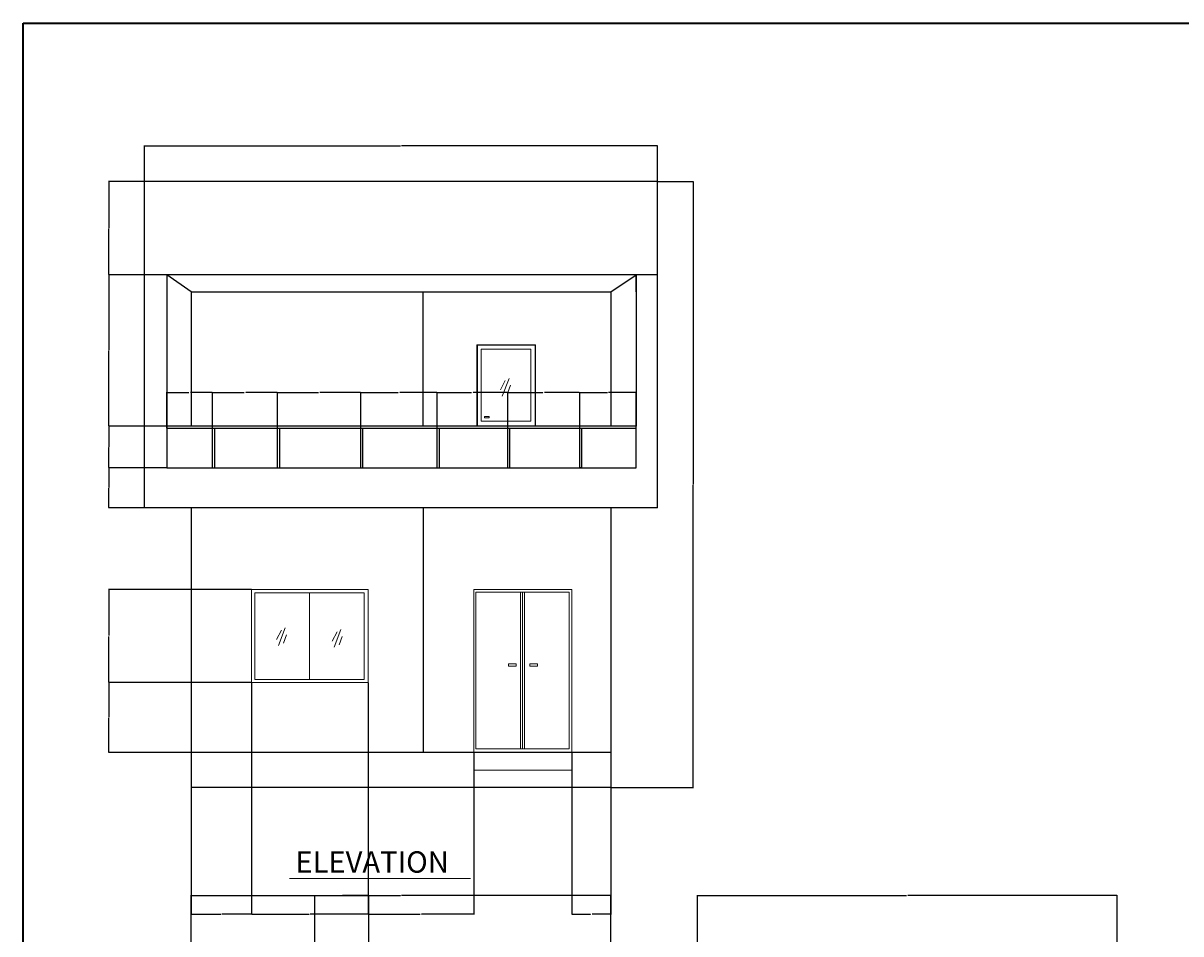
# Model space of a CAD drawing. Units: inches. Extents: x 2003 to 3241, y 1726 to 2849.
# Tile 5 of 7: x 2003 to 2599, y 2380 to 2849. Entities that reach past the tile are written whole.
import ezdxf

# ---------------------------------------------------------------- set-up
doc = ezdxf.new("R2010")
doc.units = ezdxf.units.IN
for name, color, linetype, lineweight in [('A-ANNO-DIMS', 2, 'Continuous', 18), ('A-ANNO-TEXT', 7, 'Continuous', 18), ('A-ANNO-TTLB', 7, 'Continuous', 35), ('A-DOOR', 3, 'Continuous', 18), ('A-ELEV', 7, 'Continuous', 25), ('A-FLOR-STRS', 7, 'Continuous', 18), ('A-GLAZ', 4, 'Continuous', 18)]:
    doc.layers.add(name, color=color, linetype=linetype, lineweight=lineweight)
doc.styles.get("Standard").update_dxf_attribs({"font": 'arial.ttf'})
doc.dimstyles.get("Standard").update_dxf_attribs({"dimtxt": 0.18, "dimasz": 0.18, "dimexe": 0.18, "dimexo": 0.0625, "dimgap": 0.09, "dimtad": 0, "dimtih": 1, "dimtoh": 1, "dimdec": 4, "dimzin": 0, "dimdsep": 46, "dimtxsty": 'Standard', "dimcen": 0.09, "dimadec": 0, "dimazin": 0, "dimtfac": 1, "dimtdec": 4, "dimtofl": 0, "dimtmove": 0, "dimatfit": 3, "dimfxl": 1, "dimtolj": 1, "dimtzin": 0, "dimarcsym": 0})

# ---------------------------------------------------------------- blocks, each defined once
blk = doc.blocks.new('*D64')
at = {"layer": 'A-ANNO-DIMS', "color": 0, "lineweight": -2, "transparency": 16777216}
for p, q in [((2089.78, 2369.98), (2089.78, 2399.74)), ((2089.96, 2399.56), (2197.49, 2399.56)), ((2305.6, 2399.56), (2198.07, 2399.56)), ((2305.78, 2369.98), (2305.78, 2399.74))]:
    blk.add_line(p, q, dxfattribs=at)
at = {"layer": 'A-ANNO-DIMS', "color": 0, "transparency": 16777216}
for points in [[(2089.96, 2399.59), (2089.96, 2399.53), (2089.78, 2399.56)], [(2305.6, 2399.59), (2305.6, 2399.53), (2305.78, 2399.56)]]:
    blk.add_solid(points, dxfattribs=at)
at = {"layer": 'Defpoints', "color": 0, "transparency": 16777216}
for p in [(2305.78, 2399.56), (2089.78, 2369.91), (2305.78, 2369.91)]:
    blk.add_point(p, dxfattribs=at)
at = {"layer": 'A-ANNO-DIMS', "color": 0, "transparency": 16777216, "insert": (2197.78, 2399.56), "char_height": 0.18, "attachment_point": 5}
blk.add_mtext('\\A1;216', dxfattribs=at)
blk = doc.blocks.new('*D68')
at = {"layer": 'A-ANNO-DIMS', "color": 0, "lineweight": -2, "transparency": 16777216}
for p, q in [((2153.35, 2174.54), (2153.35, 2399.74)), ((2153.53, 2399.56), (2166.88, 2399.56)), ((2181.01, 2399.56), (2167.67, 2399.56)), ((2181.19, 2174.54), (2181.19, 2399.74))]:
    blk.add_line(p, q, dxfattribs=at)
at = {"layer": 'A-ANNO-DIMS', "color": 0, "transparency": 16777216}
for points in [[(2153.53, 2399.59), (2153.53, 2399.53), (2153.35, 2399.56)], [(2181.01, 2399.59), (2181.01, 2399.53), (2181.19, 2399.56)]]:
    blk.add_solid(points, dxfattribs=at)
at = {"layer": 'Defpoints', "color": 0, "transparency": 16777216}
for p in [(2181.19, 2399.56), (2153.35, 2174.48), (2181.19, 2174.48)]:
    blk.add_point(p, dxfattribs=at)
at = {"layer": 'A-ANNO-DIMS', "color": 0, "transparency": 16777216, "insert": (2167.27, 2399.56), "char_height": 0.18, "attachment_point": 5}
blk.add_mtext('\\A1;27.84', dxfattribs=at)
blk = doc.blocks.new('*D70')
at = {"layer": 'A-ANNO-DIMS', "color": 0, "lineweight": -2, "transparency": 16777216}
for p, q in [((2350.3, 2369.98), (2350.3, 2399.74)), ((2350.48, 2399.56), (2458.01, 2399.56)), ((2566.12, 2399.56), (2458.59, 2399.56)), ((2566.3, 2369.98), (2566.3, 2399.74))]:
    blk.add_line(p, q, dxfattribs=at)
at = {"layer": 'A-ANNO-DIMS', "color": 0, "transparency": 16777216}
for points in [[(2350.48, 2399.59), (2350.48, 2399.53), (2350.3, 2399.56)], [(2566.12, 2399.59), (2566.12, 2399.53), (2566.3, 2399.56)]]:
    blk.add_solid(points, dxfattribs=at)
at = {"layer": 'Defpoints', "color": 0, "transparency": 16777216}
for p in [(2566.3, 2399.56), (2350.3, 2369.91), (2566.3, 2369.91)]:
    blk.add_point(p, dxfattribs=at)
at = {"layer": 'A-ANNO-DIMS', "color": 0, "transparency": 16777216, "insert": (2458.3, 2399.56), "char_height": 0.18, "attachment_point": 5}
blk.add_mtext('\\A1;216', dxfattribs=at)
blk = doc.blocks.new('*D81')
at = {"layer": 'A-ANNO-DIMS', "color": 0, "lineweight": -2, "transparency": 16777216}
for p, q in [((2065.78, 2767.24), (2065.78, 2785.71)), ((2065.96, 2785.53), (2197.49, 2785.53)), ((2329.6, 2785.53), (2198.07, 2785.53)), ((2329.78, 2767.24), (2329.78, 2785.71))]:
    blk.add_line(p, q, dxfattribs=at)
at = {"layer": 'A-ANNO-DIMS', "color": 0, "transparency": 16777216}
for points in [[(2065.96, 2785.56), (2065.96, 2785.5), (2065.78, 2785.53)], [(2329.6, 2785.56), (2329.6, 2785.5), (2329.78, 2785.53)]]:
    blk.add_solid(points, dxfattribs=at)
at = {"layer": 'Defpoints', "color": 0, "transparency": 16777216}
for p in [(2329.78, 2785.53), (2065.78, 2767.18), (2329.78, 2767.18)]:
    blk.add_point(p, dxfattribs=at)
at = {"layer": 'A-ANNO-DIMS', "color": 0, "transparency": 16777216, "insert": (2197.78, 2785.53), "char_height": 0.18, "attachment_point": 5}
blk.add_mtext('\\A1;264', dxfattribs=at)
blk = doc.blocks.new('*D82')
at = {"layer": 'A-ANNO-DIMS', "color": 0, "lineweight": -2, "transparency": 16777216}
for p, q in [((2329.84, 2767.18), (2348.31, 2767.18)), ((2348.13, 2767), (2348.13, 2611.36)), ((2348.13, 2455.36), (2348.13, 2611)), ((2305.84, 2455.18), (2348.31, 2455.18))]:
    blk.add_line(p, q, dxfattribs=at)
at = {"layer": 'A-ANNO-DIMS', "color": 0, "transparency": 16777216}
for points in [[(2348.1, 2767), (2348.16, 2767), (2348.13, 2767.18)], [(2348.1, 2455.36), (2348.16, 2455.36), (2348.13, 2455.18)]]:
    blk.add_solid(points, dxfattribs=at)
at = {"layer": 'Defpoints', "color": 0, "transparency": 16777216}
for p in [(2329.78, 2767.18), (2348.13, 2767.18), (2305.78, 2455.18)]:
    blk.add_point(p, dxfattribs=at)
at = {"layer": 'A-ANNO-DIMS', "color": 0, "transparency": 16777216, "insert": (2348.13, 2611.18), "char_height": 0.18, "attachment_point": 5}
blk.add_mtext('\\A1;312', dxfattribs=at)
blk = doc.blocks.new('*D83')
at = {"layer": 'A-ANNO-DIMS', "color": 0, "lineweight": -2, "transparency": 16777216}
for p, q in [((2077.13, 2619.77), (2047.25, 2619.77)), ((2047.43, 2619.59), (2047.43, 2609.66)), ((2047.43, 2599.36), (2047.43, 2609.29)), ((2065.72, 2599.18), (2047.25, 2599.18))]:
    blk.add_line(p, q, dxfattribs=at)
at = {"layer": 'A-ANNO-DIMS', "color": 0, "transparency": 16777216}
for points in [[(2047.4, 2619.59), (2047.46, 2619.59), (2047.43, 2619.77)], [(2047.4, 2599.36), (2047.46, 2599.36), (2047.43, 2599.18)]]:
    blk.add_solid(points, dxfattribs=at)
at = {"layer": 'Defpoints', "color": 0, "transparency": 16777216}
for p in [(2047.43, 2619.77), (2077.2, 2619.77), (2065.78, 2599.18)]:
    blk.add_point(p, dxfattribs=at)
at = {"layer": 'A-ANNO-DIMS', "color": 0, "transparency": 16777216, "insert": (2047.43, 2609.48), "char_height": 0.18, "attachment_point": 5}
blk.add_mtext('\\A1;20.59', dxfattribs=at)
blk = doc.blocks.new('*D84')
at = {"layer": 'A-ANNO-DIMS', "color": 0, "lineweight": -2, "transparency": 16777216}
for p, q in [((2077.13, 2641.18), (2047.25, 2641.18)), ((2047.43, 2641), (2047.43, 2630.66)), ((2047.43, 2619.95), (2047.43, 2630.3)), ((2077.13, 2619.77), (2047.25, 2619.77))]:
    blk.add_line(p, q, dxfattribs=at)
at = {"layer": 'A-ANNO-DIMS', "color": 0, "transparency": 16777216}
for points in [[(2047.4, 2641), (2047.46, 2641), (2047.43, 2641.18)], [(2047.4, 2619.95), (2047.46, 2619.95), (2047.43, 2619.77)]]:
    blk.add_solid(points, dxfattribs=at)
at = {"layer": 'Defpoints', "color": 0, "transparency": 16777216}
for p in [(2047.43, 2641.18), (2077.2, 2641.18), (2077.2, 2619.77)]:
    blk.add_point(p, dxfattribs=at)
at = {"layer": 'A-ANNO-DIMS', "color": 0, "transparency": 16777216, "insert": (2047.43, 2630.48), "char_height": 0.18, "attachment_point": 5}
blk.add_mtext('\\A1;21.41', dxfattribs=at)
blk = doc.blocks.new('*D85')
at = {"layer": 'A-ANNO-DIMS', "color": 0, "lineweight": -2, "transparency": 16777216}
for p, q in [((2065.72, 2719.18), (2047.25, 2719.18)), ((2047.43, 2719), (2047.43, 2680.36)), ((2047.43, 2641.36), (2047.43, 2680)), ((2077.13, 2641.18), (2047.25, 2641.18))]:
    blk.add_line(p, q, dxfattribs=at)
at = {"layer": 'A-ANNO-DIMS', "color": 0, "transparency": 16777216}
for points in [[(2047.4, 2719), (2047.46, 2719), (2047.43, 2719.18)], [(2047.4, 2641.36), (2047.46, 2641.36), (2047.43, 2641.18)]]:
    blk.add_solid(points, dxfattribs=at)
at = {"layer": 'Defpoints', "color": 0, "transparency": 16777216}
for p in [(2047.43, 2719.18), (2065.78, 2719.18), (2077.2, 2641.18)]:
    blk.add_point(p, dxfattribs=at)
at = {"layer": 'A-ANNO-DIMS', "color": 0, "transparency": 16777216, "insert": (2047.43, 2680.18), "char_height": 0.18, "attachment_point": 5}
blk.add_mtext('\\A1;78', dxfattribs=at)
blk = doc.blocks.new('*D86')
at = {"layer": 'A-ANNO-DIMS', "color": 0, "lineweight": -2, "transparency": 16777216}
for p, q in [((2065.72, 2767.18), (2047.25, 2767.18)), ((2047.43, 2767), (2047.43, 2743.36)), ((2047.43, 2719.36), (2047.43, 2743)), ((2065.72, 2719.18), (2047.25, 2719.18))]:
    blk.add_line(p, q, dxfattribs=at)
at = {"layer": 'A-ANNO-DIMS', "color": 0, "transparency": 16777216}
for points in [[(2047.4, 2767), (2047.46, 2767), (2047.43, 2767.18)], [(2047.4, 2719.36), (2047.46, 2719.36), (2047.43, 2719.18)]]:
    blk.add_solid(points, dxfattribs=at)
at = {"layer": 'Defpoints', "color": 0, "transparency": 16777216}
for p in [(2047.43, 2767.18), (2065.78, 2767.18), (2065.78, 2719.18)]:
    blk.add_point(p, dxfattribs=at)
at = {"layer": 'A-ANNO-DIMS', "color": 0, "transparency": 16777216, "insert": (2047.43, 2743.18), "char_height": 0.18, "attachment_point": 5}
blk.add_mtext('\\A1;48', dxfattribs=at)
blk = doc.blocks.new('*D87')
at = {"layer": 'A-ANNO-DIMS', "color": 0, "lineweight": -2, "transparency": 16777216}
for p, q in [((2077.2, 2640.24), (2077.2, 2658.71)), ((2077.38, 2658.53), (2088.54, 2658.53)), ((2100.5, 2658.53), (2089.33, 2658.53)), ((2100.68, 2640.24), (2100.68, 2658.71))]:
    blk.add_line(p, q, dxfattribs=at)
at = {"layer": 'A-ANNO-DIMS', "color": 0, "transparency": 16777216}
for points in [[(2077.38, 2658.56), (2077.38, 2658.5), (2077.2, 2658.53)], [(2100.5, 2658.56), (2100.5, 2658.5), (2100.68, 2658.53)]]:
    blk.add_solid(points, dxfattribs=at)
at = {"layer": 'Defpoints', "color": 0, "transparency": 16777216}
for p in [(2100.68, 2658.53), (2077.2, 2640.18), (2100.68, 2640.18)]:
    blk.add_point(p, dxfattribs=at)
at = {"layer": 'A-ANNO-DIMS', "color": 0, "transparency": 16777216, "insert": (2088.94, 2658.53), "char_height": 0.18, "attachment_point": 5}
blk.add_mtext('\\A1;23.48', dxfattribs=at)
blk = doc.blocks.new('*D88')
at = {"layer": 'A-ANNO-DIMS', "color": 0, "lineweight": -2, "transparency": 16777216}
for p, q in [((2100.68, 2640.24), (2100.68, 2658.71)), ((2100.86, 2658.53), (2117.07, 2658.53)), ((2134.08, 2658.53), (2117.86, 2658.53)), ((2134.26, 2640.24), (2134.26, 2658.71))]:
    blk.add_line(p, q, dxfattribs=at)
at = {"layer": 'A-ANNO-DIMS', "color": 0, "transparency": 16777216}
for points in [[(2100.86, 2658.56), (2100.86, 2658.5), (2100.68, 2658.53)], [(2134.08, 2658.56), (2134.08, 2658.5), (2134.26, 2658.53)]]:
    blk.add_solid(points, dxfattribs=at)
at = {"layer": 'Defpoints', "color": 0, "transparency": 16777216}
for p in [(2134.26, 2658.53), (2100.68, 2640.18), (2134.26, 2640.18)]:
    blk.add_point(p, dxfattribs=at)
at = {"layer": 'A-ANNO-DIMS', "color": 0, "transparency": 16777216, "insert": (2117.47, 2658.53), "char_height": 0.18, "attachment_point": 5}
blk.add_mtext('\\A1;33.58', dxfattribs=at)
blk = doc.blocks.new('*D89')
at = {"layer": 'A-ANNO-DIMS', "color": 0, "lineweight": -2, "transparency": 16777216}
for p, q in [((2134.26, 2640.24), (2134.26, 2658.71)), ((2134.44, 2658.53), (2155.23, 2658.53)), ((2176.83, 2658.53), (2156.03, 2658.53)), ((2177.01, 2640.24), (2177.01, 2658.71))]:
    blk.add_line(p, q, dxfattribs=at)
at = {"layer": 'A-ANNO-DIMS', "color": 0, "transparency": 16777216}
for points in [[(2134.44, 2658.56), (2134.44, 2658.5), (2134.26, 2658.53)], [(2176.83, 2658.56), (2176.83, 2658.5), (2177.01, 2658.53)]]:
    blk.add_solid(points, dxfattribs=at)
at = {"layer": 'Defpoints', "color": 0, "transparency": 16777216}
for p in [(2177.01, 2658.53), (2134.26, 2640.18), (2177.01, 2640.18)]:
    blk.add_point(p, dxfattribs=at)
at = {"layer": 'A-ANNO-DIMS', "color": 0, "transparency": 16777216, "insert": (2155.63, 2658.53), "char_height": 0.18, "attachment_point": 5}
blk.add_mtext('\\A1;42.75', dxfattribs=at)
blk = doc.blocks.new('*D90')
at = {"layer": 'A-ANNO-DIMS', "color": 0, "lineweight": -2, "transparency": 16777216}
for p, q in [((2177.01, 2640.24), (2177.01, 2658.71)), ((2177.19, 2658.53), (2196.2, 2658.53)), ((2216.13, 2658.53), (2197.12, 2658.53)), ((2216.31, 2640.24), (2216.31, 2658.71))]:
    blk.add_line(p, q, dxfattribs=at)
at = {"layer": 'A-ANNO-DIMS', "color": 0, "transparency": 16777216}
for points in [[(2177.19, 2658.56), (2177.19, 2658.5), (2177.01, 2658.53)], [(2216.13, 2658.56), (2216.13, 2658.5), (2216.31, 2658.53)]]:
    blk.add_solid(points, dxfattribs=at)
at = {"layer": 'Defpoints', "color": 0, "transparency": 16777216}
for p in [(2216.31, 2658.53), (2177.01, 2640.18), (2216.31, 2640.18)]:
    blk.add_point(p, dxfattribs=at)
at = {"layer": 'A-ANNO-DIMS', "color": 0, "transparency": 16777216, "insert": (2196.66, 2658.53), "char_height": 0.18, "attachment_point": 5}
blk.add_mtext('\\A1;39.304', dxfattribs=at)
blk = doc.blocks.new('*D91')
at = {"layer": 'A-ANNO-DIMS', "color": 0, "lineweight": -2, "transparency": 16777216}
for p, q in [((2216.31, 2640.24), (2216.31, 2658.71)), ((2216.49, 2658.53), (2234.09, 2658.53)), ((2252.48, 2658.53), (2234.88, 2658.53)), ((2252.66, 2640.24), (2252.66, 2658.71))]:
    blk.add_line(p, q, dxfattribs=at)
at = {"layer": 'A-ANNO-DIMS', "color": 0, "transparency": 16777216}
for points in [[(2216.49, 2658.56), (2216.49, 2658.5), (2216.31, 2658.53)], [(2252.48, 2658.56), (2252.48, 2658.5), (2252.66, 2658.53)]]:
    blk.add_solid(points, dxfattribs=at)
at = {"layer": 'Defpoints', "color": 0, "transparency": 16777216}
for p in [(2252.66, 2658.53), (2216.31, 2640.18), (2252.66, 2640.18)]:
    blk.add_point(p, dxfattribs=at)
at = {"layer": 'A-ANNO-DIMS', "color": 0, "transparency": 16777216, "insert": (2234.49, 2658.53), "char_height": 0.18, "attachment_point": 5}
blk.add_mtext('\\A1;36.35', dxfattribs=at)
blk = doc.blocks.new('*D92')
at = {"layer": 'A-ANNO-DIMS', "color": 0, "lineweight": -2, "transparency": 16777216}
for p, q in [((2252.66, 2640.24), (2252.66, 2658.71)), ((2252.84, 2658.53), (2270.79, 2658.53)), ((2289.53, 2658.53), (2271.58, 2658.53)), ((2289.71, 2640.24), (2289.71, 2658.71))]:
    blk.add_line(p, q, dxfattribs=at)
at = {"layer": 'A-ANNO-DIMS', "color": 0, "transparency": 16777216}
for points in [[(2252.84, 2658.56), (2252.84, 2658.5), (2252.66, 2658.53)], [(2289.53, 2658.56), (2289.53, 2658.5), (2289.71, 2658.53)]]:
    blk.add_solid(points, dxfattribs=at)
at = {"layer": 'Defpoints', "color": 0, "transparency": 16777216}
for p in [(2289.71, 2658.53), (2252.66, 2640.18), (2289.71, 2640.18)]:
    blk.add_point(p, dxfattribs=at)
at = {"layer": 'A-ANNO-DIMS', "color": 0, "transparency": 16777216, "insert": (2271.19, 2658.53), "char_height": 0.18, "attachment_point": 5}
blk.add_mtext('\\A1;37.04', dxfattribs=at)
blk = doc.blocks.new('*D93')
at = {"layer": 'A-ANNO-DIMS', "color": 0, "lineweight": -2, "transparency": 16777216}
for p, q in [((2289.71, 2640.24), (2289.71, 2658.71)), ((2289.89, 2658.53), (2303.95, 2658.53)), ((2318.63, 2658.53), (2304.56, 2658.53)), ((2318.81, 2640.24), (2318.81, 2658.71))]:
    blk.add_line(p, q, dxfattribs=at)
at = {"layer": 'A-ANNO-DIMS', "color": 0, "transparency": 16777216}
for points in [[(2289.89, 2658.56), (2289.89, 2658.5), (2289.71, 2658.53)], [(2318.63, 2658.56), (2318.63, 2658.5), (2318.81, 2658.53)]]:
    blk.add_solid(points, dxfattribs=at)
at = {"layer": 'Defpoints', "color": 0, "transparency": 16777216}
for p in [(2318.81, 2658.53), (2289.71, 2640.18), (2318.81, 2640.18)]:
    blk.add_point(p, dxfattribs=at)
at = {"layer": 'A-ANNO-DIMS', "color": 0, "transparency": 16777216, "insert": (2304.26, 2658.53), "char_height": 0.18, "attachment_point": 5}
blk.add_mtext('\\A1;29.1', dxfattribs=at)
blk = doc.blocks.new('*D94')
at = {"layer": 'A-ANNO-DIMS', "color": 0, "lineweight": -2, "transparency": 16777216}
for p, q in [((2120.78, 2509.12), (2120.78, 2389.73)), ((2089.78, 2455.12), (2089.78, 2389.73)), ((2089.96, 2389.91), (2105.08, 2389.91)), ((2120.6, 2389.91), (2105.48, 2389.91))]:
    blk.add_line(p, q, dxfattribs=at)
at = {"layer": 'A-ANNO-DIMS', "color": 0, "transparency": 16777216}
for points in [[(2089.96, 2389.94), (2089.96, 2389.88), (2089.78, 2389.91)], [(2120.6, 2389.94), (2120.6, 2389.88), (2120.78, 2389.91)]]:
    blk.add_solid(points, dxfattribs=at)
at = {"layer": 'Defpoints', "color": 0, "transparency": 16777216}
for p in [(2120.78, 2509.18), (2089.78, 2455.18), (2120.78, 2389.91)]:
    blk.add_point(p, dxfattribs=at)
at = {"layer": 'A-ANNO-DIMS', "color": 0, "transparency": 16777216, "insert": (2105.28, 2389.91), "char_height": 0.18, "attachment_point": 5}
blk.add_mtext('\\A1;31', dxfattribs=at)
blk = doc.blocks.new('*D95')
at = {"layer": 'A-ANNO-DIMS', "color": 0, "lineweight": -2, "transparency": 16777216}
for p, q in [((2120.78, 2509.12), (2120.78, 2389.73)), ((2180.78, 2509.12), (2180.78, 2389.73)), ((2120.96, 2389.91), (2150.56, 2389.91)), ((2180.6, 2389.91), (2151, 2389.91))]:
    blk.add_line(p, q, dxfattribs=at)
at = {"layer": 'A-ANNO-DIMS', "color": 0, "transparency": 16777216}
for points in [[(2120.96, 2389.94), (2120.96, 2389.88), (2120.78, 2389.91)], [(2180.6, 2389.94), (2180.6, 2389.88), (2180.78, 2389.91)]]:
    blk.add_solid(points, dxfattribs=at)
at = {"layer": 'Defpoints', "color": 0, "transparency": 16777216}
for p in [(2120.78, 2509.18), (2180.78, 2509.18), (2180.78, 2389.91)]:
    blk.add_point(p, dxfattribs=at)
at = {"layer": 'A-ANNO-DIMS', "color": 0, "transparency": 16777216, "insert": (2150.78, 2389.91), "char_height": 0.18, "attachment_point": 5}
blk.add_mtext('\\A1;60', dxfattribs=at)
blk = doc.blocks.new('*D96')
at = {"layer": 'A-ANNO-DIMS', "color": 0, "lineweight": -2, "transparency": 16777216}
for p, q in [((2180.78, 2509.12), (2180.78, 2389.73)), ((2235.19, 2473.12), (2235.19, 2389.73)), ((2180.96, 2389.91), (2207.61, 2389.91)), ((2235.01, 2389.91), (2208.36, 2389.91))]:
    blk.add_line(p, q, dxfattribs=at)
at = {"layer": 'A-ANNO-DIMS', "color": 0, "transparency": 16777216}
for points in [[(2180.96, 2389.94), (2180.96, 2389.88), (2180.78, 2389.91)], [(2235.01, 2389.94), (2235.01, 2389.88), (2235.19, 2389.91)]]:
    blk.add_solid(points, dxfattribs=at)
at = {"layer": 'Defpoints', "color": 0, "transparency": 16777216}
for p in [(2180.78, 2509.18), (2235.19, 2473.18), (2235.19, 2389.91)]:
    blk.add_point(p, dxfattribs=at)
at = {"layer": 'A-ANNO-DIMS', "color": 0, "transparency": 16777216, "insert": (2207.99, 2389.91), "char_height": 0.18, "attachment_point": 5}
blk.add_mtext('\\A1;54.41', dxfattribs=at)
blk = doc.blocks.new('*D97')
at = {"layer": 'A-ANNO-DIMS', "color": 0, "lineweight": -2, "transparency": 16777216}
for p, q in [((2285.67, 2473.12), (2285.67, 2389.73)), ((2305.78, 2455.12), (2305.78, 2389.73)), ((2285.85, 2389.91), (2295.26, 2389.91)), ((2305.6, 2389.91), (2296.19, 2389.91))]:
    blk.add_line(p, q, dxfattribs=at)
at = {"layer": 'A-ANNO-DIMS', "color": 0, "transparency": 16777216}
for points in [[(2285.85, 2389.94), (2285.85, 2389.88), (2285.67, 2389.91)], [(2305.6, 2389.94), (2305.6, 2389.88), (2305.78, 2389.91)]]:
    blk.add_solid(points, dxfattribs=at)
at = {"layer": 'Defpoints', "color": 0, "transparency": 16777216}
for p in [(2285.67, 2473.18), (2305.78, 2455.18), (2305.78, 2389.91)]:
    blk.add_point(p, dxfattribs=at)
at = {"layer": 'A-ANNO-DIMS', "color": 0, "transparency": 16777216, "insert": (2295.72, 2389.91), "char_height": 0.18, "attachment_point": 5}
blk.add_mtext('\\A1;20.108', dxfattribs=at)
blk = doc.blocks.new('*D98')
at = {"layer": 'A-ANNO-DIMS', "color": 0, "lineweight": -2, "transparency": 16777216}
for p, q in [((2120.72, 2509.18), (2047.25, 2509.18)), ((2047.43, 2509), (2047.43, 2491.36)), ((2047.43, 2473.36), (2047.43, 2491)), ((2089.72, 2473.18), (2047.25, 2473.18))]:
    blk.add_line(p, q, dxfattribs=at)
at = {"layer": 'A-ANNO-DIMS', "color": 0, "transparency": 16777216}
for points in [[(2047.4, 2509), (2047.46, 2509), (2047.43, 2509.18)], [(2047.4, 2473.36), (2047.46, 2473.36), (2047.43, 2473.18)]]:
    blk.add_solid(points, dxfattribs=at)
at = {"layer": 'Defpoints', "color": 0, "transparency": 16777216}
for p in [(2047.43, 2509.18), (2120.78, 2509.18), (2089.78, 2473.18)]:
    blk.add_point(p, dxfattribs=at)
at = {"layer": 'A-ANNO-DIMS', "color": 0, "transparency": 16777216, "insert": (2047.43, 2491.18), "char_height": 0.18, "attachment_point": 5}
blk.add_mtext('\\A1;36', dxfattribs=at)
blk = doc.blocks.new('*D99')
at = {"layer": 'A-ANNO-DIMS', "color": 0, "lineweight": -2, "transparency": 16777216}
for p, q in [((2120.72, 2557.18), (2047.25, 2557.18)), ((2047.43, 2557), (2047.43, 2533.36)), ((2047.43, 2509.36), (2047.43, 2533)), ((2120.72, 2509.18), (2047.25, 2509.18))]:
    blk.add_line(p, q, dxfattribs=at)
at = {"layer": 'A-ANNO-DIMS', "color": 0, "transparency": 16777216}
for points in [[(2047.4, 2557), (2047.46, 2557), (2047.43, 2557.18)], [(2047.4, 2509.36), (2047.46, 2509.36), (2047.43, 2509.18)]]:
    blk.add_solid(points, dxfattribs=at)
at = {"layer": 'Defpoints', "color": 0, "transparency": 16777216}
for p in [(2047.43, 2557.18), (2120.78, 2557.18), (2120.78, 2509.18)]:
    blk.add_point(p, dxfattribs=at)
at = {"layer": 'A-ANNO-DIMS', "color": 0, "transparency": 16777216, "insert": (2047.43, 2533.18), "char_height": 0.18, "attachment_point": 5}
blk.add_mtext('\\A1;48', dxfattribs=at)

msp = doc.modelspace()

# ---------------------------------------------------------------- linework, layer by layer
at = {"layer": 'A-ANNO-TEXT'}
msp.add_line((2140.3445, 2408.2607), (2233.4534, 2408.2607), dxfattribs=at)
at = {"layer": 'A-ANNO-TTLB'}
msp.add_lwpolyline([(2003.2633, 2848.7261), (3241.1194, 2848.7261), (3241.1194, 1726.227), (2003.2633, 1726.227)], close=True, dxfattribs=at)
at = {"layer": 'A-DOOR'}
for p, q in [((2236.7095, 2683.181), (2236.7095, 2641.181)), ((2266.9682, 2683.181), (2236.7095, 2683.181)), ((2266.9682, 2683.181), (2266.9682, 2641.181)), ((2251.4119, 2664.7024), (2248.8765, 2659.9434)), ((2253.3462, 2665.8437), (2249.8975, 2656.7228)), ((2254.0882, 2662.337), (2252.5106, 2658.0004)), ((2235.1913, 2557.181), (2235.1913, 2473.181)), ((2285.6705, 2557.181), (2235.1913, 2557.181)), ((2285.6705, 2557.181), (2285.6705, 2473.181)), ((2259.3161, 2475.0768), (2259.3161, 2555.7453)), ((2259.3161, 2555.7453), (2260.3161, 2555.7453)), ((2260.3161, 2555.7453), (2260.3161, 2475.0768)), ((2260.3161, 2555.7453), (2261.3161, 2555.7453)), ((2261.3161, 2555.7453), (2261.3161, 2475.0768)), ((2260.3161, 2475.0768), (2259.3161, 2475.0768))]:
    msp.add_line(p, q, dxfattribs=at)
for points in [[(2237.0441, 2682.8641), (2266.7587, 2682.8641), (2266.7587, 2641.181), (2237.0441, 2641.181)], [(2239.0779, 2680.8556), (2264.6435, 2680.8556), (2264.6435, 2643.8128), (2239.0779, 2643.8128)], [(2240.6371, 2646.1999), (2243.1393, 2646.1999), (2243.1393, 2645.5867), (2240.6371, 2645.5867)], [(2236.2879, 2555.7453), (2284.3444, 2555.7453), (2284.3444, 2475.0768), (2236.2879, 2475.0768)], [(2253.0229, 2518.8672), (2256.9766, 2518.8672), (2256.9766, 2517.6705), (2253.0229, 2517.6705)], [(2264.091, 2518.8672), (2268.0446, 2518.8672), (2268.0446, 2517.6705), (2264.091, 2517.6705)]]:
    msp.add_lwpolyline(points, close=True, dxfattribs=at)
at = {"layer": 'A-ELEV'}
for p, q in [((2329.7784, 2767.181), (2065.7784, 2767.181)), ((2065.7784, 2599.181), (2065.7784, 2767.181)), ((2329.7784, 2599.181), (2329.7784, 2767.181)), ((2329.7784, 2719.181), (2065.7784, 2719.181)), ((2077.1959, 2719.181), (2077.1959, 2641.181)), ((2089.7784, 2710.4171), (2077.1959, 2719.181)), ((2305.7784, 2710.4171), (2318.8074, 2719.181)), ((2318.8074, 2710.4171), (2318.8074, 2719.181)), ((2318.8074, 2719.181), (2318.8074, 2641.181)), ((2089.7784, 2710.4171), (2089.7784, 2641.181)), ((2089.7784, 2710.4171), (2305.7784, 2710.4171)), ((2209.1571, 2641.181), (2209.1571, 2710.4171)), ((2305.7784, 2710.4171), (2305.7784, 2641.181)), ((2318.8074, 2641.181), (2077.1959, 2641.181)), ((2077.1959, 2641.181), (2077.1959, 2619.7719)), ((2077.1959, 2641.181), (2077.1959, 2640.181)), ((2077.1959, 2640.181), (2318.8074, 2640.181)), ((2100.6782, 2619.7719), (2100.6782, 2640.181)), ((2101.6782, 2640.181), (2101.6782, 2619.7719)), ((2134.2555, 2619.7719), (2134.2555, 2640.181)), ((2135.2555, 2640.181), (2135.2555, 2619.7719)), ((2177.0084, 2619.7719), (2177.0084, 2640.181)), ((2178.0084, 2640.181), (2178.0084, 2619.7719)), ((2216.3128, 2619.7719), (2216.3128, 2640.181)), ((2217.3128, 2640.181), (2217.3128, 2619.7719)), ((2252.6647, 2619.7719), (2252.6647, 2640.181)), ((2253.6647, 2640.181), (2253.6647, 2619.7719)), ((2289.7054, 2619.7719), (2289.7054, 2640.181)), ((2290.7054, 2640.181), (2290.7054, 2619.7719)), ((2318.8074, 2619.7719), (2318.8074, 2641.181)), ((2077.1959, 2619.7719), (2318.8074, 2619.7719)), ((2290.7054, 2619.7719), (2289.7054, 2619.7719)), ((2329.7784, 2599.181), (2065.7784, 2599.181)), ((2089.7784, 2599.181), (2089.7784, 2455.181)), ((2089.7784, 2599.181), (2089.7784, 2581.181)), ((2209.142, 2599.181), (2209.142, 2473.181)), ((2305.7784, 2599.181), (2305.7784, 2455.181)), ((2305.7784, 2599.181), (2305.7784, 2581.181)), ((2305.7784, 2473.181), (2089.7784, 2473.181)), ((2305.7784, 2455.181), (2089.7784, 2455.181))]:
    msp.add_line(p, q, dxfattribs=at)
at = {"layer": 'A-FLOR-STRS'}
for p, q in [((2235.1913, 2473.181), (2235.1913, 2455.181)), ((2285.6705, 2473.181), (2285.6705, 2455.181)), ((2285.6705, 2464.181), (2235.1913, 2464.181)), ((2285.6705, 2455.181), (2285.6705, 2464.181))]:
    msp.add_line(p, q, dxfattribs=at)
at = {"layer": 'A-GLAZ'}
for p, q in [((2120.7798, 2557.181), (2120.7798, 2509.181)), ((2180.7798, 2557.181), (2120.7798, 2557.181)), ((2180.7798, 2557.181), (2180.7798, 2509.181)), ((2150.6517, 2555.4541), (2150.6517, 2510.8475)), ((2136.1838, 2536.2096), (2133.6484, 2531.4506)), ((2138.1181, 2537.3508), (2134.6694, 2528.2299)), ((2138.8601, 2533.8441), (2137.2825, 2529.5075)), ((2164.8399, 2535.3345), (2162.3045, 2530.5754)), ((2166.7742, 2536.4757), (2163.3255, 2527.3548)), ((2167.5162, 2532.969), (2165.9386, 2528.6324)), ((2180.7798, 2509.181), (2120.7798, 2509.181))]:
    msp.add_line(p, q, dxfattribs=at)
msp.add_lwpolyline([(2122.4671, 2555.4541), (2178.8363, 2555.4541), (2178.8363, 2510.8475), (2122.4671, 2510.8475)], close=True, dxfattribs=at)

# ---------------------------------------------------------------- texts
at = {"layer": 'A-ANNO-TEXT', "insert": (2143.4129, 2422.3146), "char_height": 11, "attachment_point": 1}
msp.add_mtext_dynamic_manual_height_columns('ELEVATION', width=150.618676, gutter_width=12.5, heights=[0], dxfattribs=at)

# ---------------------------------------------------------------- dimensions: what is measured, and where the dimension line sits
at = {"layer": 'A-ANNO-DIMS'}
for base, p1, p2, override, picture, middle in [((2329.7784, 2785.531), (2065.7784, 2767.181), (2329.7784, 2767.181), {"dimdec": 0, "dimlfac": 1, "dimrnd": 0, "dimzin": 0, "dimdsep": 46, "dimlunit": 2}, '*D81', (2197.7784, 2785.531)), ((2100.6782, 2658.531), (2077.1959, 2640.181), (2100.6782, 2640.181), {"dimdec": 2, "dimlfac": 1, "dimrnd": 0, "dimzin": 0, "dimdsep": 46, "dimlunit": 2}, '*D87', (2088.937, 2658.531)), ((2134.2555, 2658.531), (2100.6782, 2640.181), (2134.2555, 2640.181), {"dimdec": 2, "dimlfac": 1, "dimrnd": 0, "dimzin": 0, "dimdsep": 46, "dimlunit": 2}, '*D88', (2117.4668, 2658.531)), ((2177.0084, 2658.531), (2134.2555, 2640.181), (2177.0084, 2640.181), {"dimdec": 2, "dimlfac": 1, "dimrnd": 0, "dimzin": 0, "dimdsep": 46, "dimlunit": 2}, '*D89', (2155.632, 2658.531)), ((2216.3128, 2658.531), (2177.0084, 2640.181), (2216.3128, 2640.181), {"dimdec": 3, "dimlfac": 1, "dimrnd": 0, "dimzin": 0, "dimdsep": 46, "dimlunit": 2}, '*D90', (2196.6606, 2658.531)), ((2252.6647, 2658.531), (2216.3128, 2640.181), (2252.6647, 2640.181), {"dimdec": 2, "dimlfac": 1, "dimrnd": 0, "dimzin": 0, "dimdsep": 46, "dimlunit": 2}, '*D91', (2234.4887, 2658.531)), ((2289.7054, 2658.531), (2252.6647, 2640.181), (2289.7054, 2640.181), {"dimdec": 2, "dimlfac": 1, "dimrnd": 0, "dimzin": 0, "dimdsep": 46, "dimlunit": 2}, '*D92', (2271.185, 2658.531)), ((2318.8074, 2658.531), (2289.7054, 2640.181), (2318.8074, 2640.181), {"dimdec": 1, "dimlfac": 1, "dimrnd": 0, "dimzin": 0, "dimdsep": 46, "dimlunit": 2}, '*D93', (2304.2564, 2658.531)), ((2120.7798, 2389.9107), (2089.7784, 2455.181), (2120.7798, 2509.181), {"dimdec": 0, "dimlfac": 1, "dimrnd": 0, "dimzin": 0, "dimdsep": 46, "dimlunit": 2}, '*D94', (2105.2791, 2389.9107)), ((2180.7798, 2389.9107), (2120.7798, 2509.181), (2180.7798, 2509.181), {"dimdec": 0, "dimlfac": 1, "dimrnd": 0, "dimzin": 0, "dimdsep": 46, "dimlunit": 2}, '*D95', (2150.7798, 2389.9107)), ((2235.1913, 2389.9107), (2180.7798, 2509.181), (2235.1913, 2473.181), {"dimdec": 2, "dimlfac": 1, "dimrnd": 0, "dimzin": 0, "dimdsep": 46, "dimlunit": 2}, '*D96', (2207.9856, 2389.9107)), ((2305.7784, 2389.9107), (2285.6705, 2473.181), (2305.7784, 2455.181), {"dimdec": 3, "dimlfac": 1, "dimrnd": 0, "dimzin": 0, "dimdsep": 46, "dimlunit": 2}, '*D97', (2295.7244, 2389.9107)), ((2305.7784, 2399.5635), (2089.7784, 2369.9135), (2305.7784, 2369.9135), {"dimdec": 0, "dimlfac": 1, "dimrnd": 0, "dimzin": 0, "dimdsep": 46, "dimlunit": 2}, '*D64', (2197.7784, 2399.5635)), ((2181.1916, 2399.5635), (2153.3538, 2174.4819), (2181.1916, 2174.4819), {"dimdec": 2, "dimlfac": 1, "dimrnd": 0, "dimzin": 0, "dimdsep": 46, "dimlunit": 2}, '*D68', (2167.2727, 2399.5635)), ((2566.3008, 2399.5635), (2350.3008, 2369.9135), (2566.3008, 2369.9135), {"dimdec": 0, "dimlfac": 1, "dimrnd": 0, "dimzin": 0, "dimdsep": 46, "dimlunit": 2}, '*D70', (2458.3008, 2399.5635))]:
    dim = msp.add_linear_dim(base=base, p1=p1, p2=p2, dimstyle='Standard', override=override, dxfattribs=at)
    dim.commit()
    dim.dimension.update_dxf_attribs({"geometry": picture, "text_midpoint": middle})
for base, p1, p2, override, picture, middle in [((2047.4284, 2767.181), (2065.7784, 2719.181), (2065.7784, 2767.181), {"dimdec": 0, "dimlfac": 1, "dimrnd": 0, "dimzin": 0, "dimdsep": 46, "dimlunit": 2}, '*D86', (2047.4284, 2743.181)), ((2348.1284, 2767.181), (2305.7784, 2455.181), (2329.7784, 2767.181), {"dimdec": 0, "dimlfac": 1, "dimrnd": 0, "dimzin": 0, "dimdsep": 46, "dimlunit": 2}, '*D82', (2348.1284, 2611.181)), ((2047.4284, 2719.181), (2077.1959, 2641.181), (2065.7784, 2719.181), {"dimdec": 0, "dimlfac": 1, "dimrnd": 0, "dimzin": 0, "dimdsep": 46, "dimlunit": 2}, '*D85', (2047.4284, 2680.181)), ((2047.4284, 2641.181), (2077.1959, 2619.7719), (2077.1959, 2641.181), {"dimdec": 2, "dimlfac": 1, "dimrnd": 0, "dimzin": 0, "dimdsep": 46, "dimlunit": 2}, '*D84', (2047.4284, 2630.4764)), ((2047.4284, 2619.7719), (2065.7784, 2599.181), (2077.1959, 2619.7719), {"dimdec": 2, "dimlfac": 1, "dimrnd": 0, "dimzin": 0, "dimdsep": 46, "dimlunit": 2}, '*D83', (2047.4284, 2609.4764)), ((2047.4284, 2557.181), (2120.7798, 2509.181), (2120.7798, 2557.181), {"dimdec": 0, "dimlfac": 1, "dimrnd": 0, "dimzin": 0, "dimdsep": 46, "dimlunit": 2}, '*D99', (2047.4284, 2533.181)), ((2047.4284, 2509.181), (2089.7784, 2473.181), (2120.7798, 2509.181), {"dimdec": 0, "dimlfac": 1, "dimrnd": 0, "dimzin": 0, "dimdsep": 46, "dimlunit": 2}, '*D98', (2047.4284, 2491.181))]:
    dim = msp.add_linear_dim(base=base, p1=p1, p2=p2, angle=90, dimstyle='Standard', override=override, dxfattribs=at)
    dim.commit()
    dim.dimension.update_dxf_attribs({"geometry": picture, "text_midpoint": middle})

doc.saveas('drawing.dxf')
